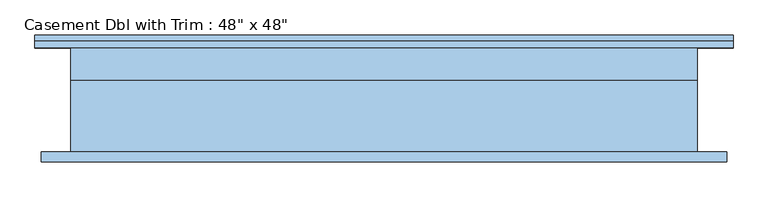
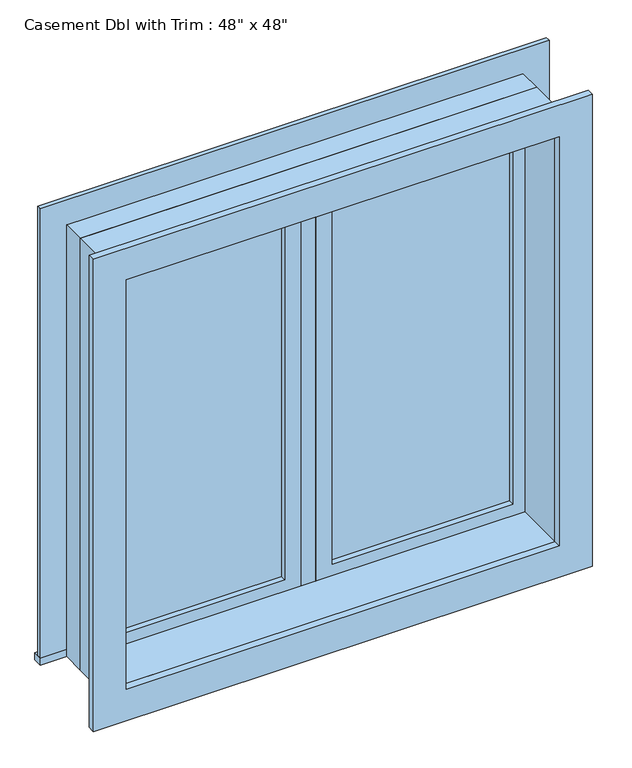
"""IFC4 building model written with IfcOpenShell, lengths in millimetres: window geometry."""

from ifc_helpers import new_model, si_unit, frame, origin, place, context, project, spatial, polyline, outline, extrude, source, transform, mapped, element, save


def window_0862ab64(model_context):
    return source(origin(), model_context, "Body", "SweptSolid", [
        extrude(outline(polyline([(63.5, 85.725), (546.1, 85.725), (546.1, 73.025), (63.5, 73.025), (63.5, 85.725)])), frame((0.0, 0.0, 977.9), z_axis=(0.0, 0.0, 1.0), x_axis=(1.0, 0.0, 0.0)), (0.0, 0.0, 1.0), 1092.2),
        extrude(outline(polyline([(2114.55, 19.05), (933.45, 19.05), (933.45, 590.55), (2114.55, 590.55), (2114.55, 19.05)]), holes=[polyline([(2070.1, 63.5), (2070.1, 546.1), (977.9, 546.1), (977.9, 63.5), (2070.1, 63.5)])]), frame((0.0, 57.15, 0.0), z_axis=(0.0, 1.0, 0.0), x_axis=(0.0, 0.0, 1.0)), (0.0, 0.0, 1.0), 44.45),
        extrude(outline(polyline([(19.05, 57.15), (-19.05, 57.15), (-19.05, 120.65), (19.05, 120.65), (19.05, 57.15)])), frame((0.0, 0.0, 933.45), z_axis=(0.0, 0.0, 1.0), x_axis=(1.0, 0.0, 0.0)), (0.0, 0.0, 1.0), 1181.1),
        extrude(outline(polyline([(-679.45, 146.05), (679.45, 146.05), (679.45, 120.65), (-679.45, 120.65), (-679.45, 146.05)])), frame((0.0, 0.0, 914.4), z_axis=(0.0, 0.0, 1.0), x_axis=(1.0, 0.0, 0.0)), (0.0, 0.0, 1.0), 19.05),
        extrude(outline(polyline([(2114.55, -590.55), (2114.55, 590.55), (933.45, 590.55), (933.45, 679.45), (2203.45, 679.45), (2203.45, -679.45), (933.45, -679.45), (933.45, -590.55), (2114.55, -590.55)])), frame((0.0, 120.65, 0.0), z_axis=(0.0, 1.0, 0.0), x_axis=(0.0, 0.0, 1.0)), (0.0, 0.0, 1.0), 12.7),
        extrude(outline(polyline([(2190.75, 666.75), (2190.75, -666.75), (857.25, -666.75), (857.25, 666.75), (2190.75, 666.75)]), holes=[polyline([(2101.85, 577.85), (946.15, 577.85), (946.15, -577.85), (2101.85, -577.85), (2101.85, 577.85)])]), frame((0.0, -101.6, 0.0), z_axis=(0.0, 1.0, 0.0), x_axis=(0.0, 0.0, 1.0)), (0.0, 0.0, 1.0), 19.05),
        extrude(outline(polyline([(-63.5, 73.025), (-546.1, 73.025), (-546.1, 85.725), (-63.5, 85.725), (-63.5, 73.025)])), frame((0.0, 0.0, 977.9), z_axis=(0.0, 0.0, 1.0), x_axis=(1.0, 0.0, 0.0)), (0.0, 0.0, 1.0), 1092.2),
        extrude(outline(polyline([(2114.55, -590.55), (933.45, -590.55), (933.45, -19.05), (2114.55, -19.05), (2114.55, -590.55)]), holes=[polyline([(2070.1, -546.1), (2070.1, -63.5), (977.9, -63.5), (977.9, -546.1), (2070.1, -546.1)])]), frame((0.0, 57.15, 0.0), z_axis=(0.0, 1.0, 0.0), x_axis=(0.0, 0.0, 1.0)), (0.0, 0.0, 1.0), 44.45),
        extrude(outline(polyline([(2133.6, -609.6), (914.4, -609.6), (914.4, 609.6), (2133.6, 609.6), (2133.6, -609.6)]), holes=[polyline([(2101.85, -577.85), (2101.85, 577.85), (946.15, 577.85), (946.15, -577.85), (2101.85, -577.85)])]), frame((0.0, -82.55, 0.0), z_axis=(0.0, 1.0, 0.0), x_axis=(0.0, 0.0, 1.0)), (0.0, 0.0, 1.0), 139.7),
        extrude(outline(polyline([(2133.6, 609.6), (2133.6, -609.6), (914.4, -609.6), (914.4, 609.6), (2133.6, 609.6)]), holes=[polyline([(2114.55, 590.55), (933.45, 590.55), (933.45, -590.55), (2114.55, -590.55), (2114.55, 590.55)])]), frame((0.0, 57.15, 0.0), z_axis=(0.0, 1.0, 0.0), x_axis=(0.0, 0.0, 1.0)), (0.0, 0.0, 1.0), 63.5),
    ])


if __name__ == "__main__":
    model = new_model("IFC4")
    model_context = context("Model", 3, world=origin())
    ifc_project = project(units=[si_unit("LENGTHUNIT", "METRE", prefix="MILLI")], contexts=[model_context])
    site = spatial("IfcSite", under=ifc_project)
    building = spatial("IfcBuilding", under=site)
    placement = place(None, origin())
    window_shape = window_0862ab64(model_context)
    element("IfcWindow", 1, ObjectType="Casement Dbl with Trim : 48\" x 48\"", at=placement, inside=building, context=model_context, shape_type="MappedRepresentation", body=[
        mapped(window_shape, transform((0.0, 0.0, 0.0), x_axis=(1.0, 0.0, 0.0), y_axis=(0.0, 1.0, 0.0), z_axis=(0.0, 0.0, 1.0))),
    ])
    save(model, "model.ifc")

# Revit data of these elements
# Type "Casement Dbl with Trim : 48\" x 48\""
#   Type Mark = "10"
#   Construction Type Id = "GSP4R"
#   Assembly Code = "B2020100"
#   Analytic Construction = "1/8 in Pilkington single glazing"
#   Visual Light Transmittance = 0.9
#   Solar Heat Gain Coefficient = 0.78
#   Heat Transfer Coefficient (U) = 0.6496 BTU/(h·ft²·°F)
#   Height = 4' - 0"
#   Default Sill Height = 3' - 0"
#   Trim Projection - Ext. = 0' - 0 1/2"
#   Trim Projection - Int. = 0' - 0 3/4"
#   Trim Width - Exterior = 0' - 3 1/2"
#   Trim Width - Interior = 0' - 3 1/2"
#   Width = 4' - 0"
#   Window Inset = 0' - 0 3/4"
#   Define Thermal Properties by = 1
#   Glass Pane Material = Glass
#   Sash Material = Glass
#   Trim Exterior Material = Glass, Clear Glazing
#   Trim Interior Material = Trim
#   Wall Closure = (empty or 0)
# Element 1 (IfcWindow, "Casement Dbl with Trim : 48\" x 48\"")
#   Materials on its faces: "Glass", "Glass, Clear Glazing", "Trim"
# Materials
#   "Glass": class "Glass", colour RGB 0 128 192, transparency 0.75, Description = "Soda Lime Glass", Cost = 0
#   "Glass, Clear Glazing": class "Glass", colour RGB 0 128 192, transparency 0.75, Description = "Clear glazing", Cost = 0
#   "Trim": class "Wood", colour RGB 224 178 126, transparency 0
